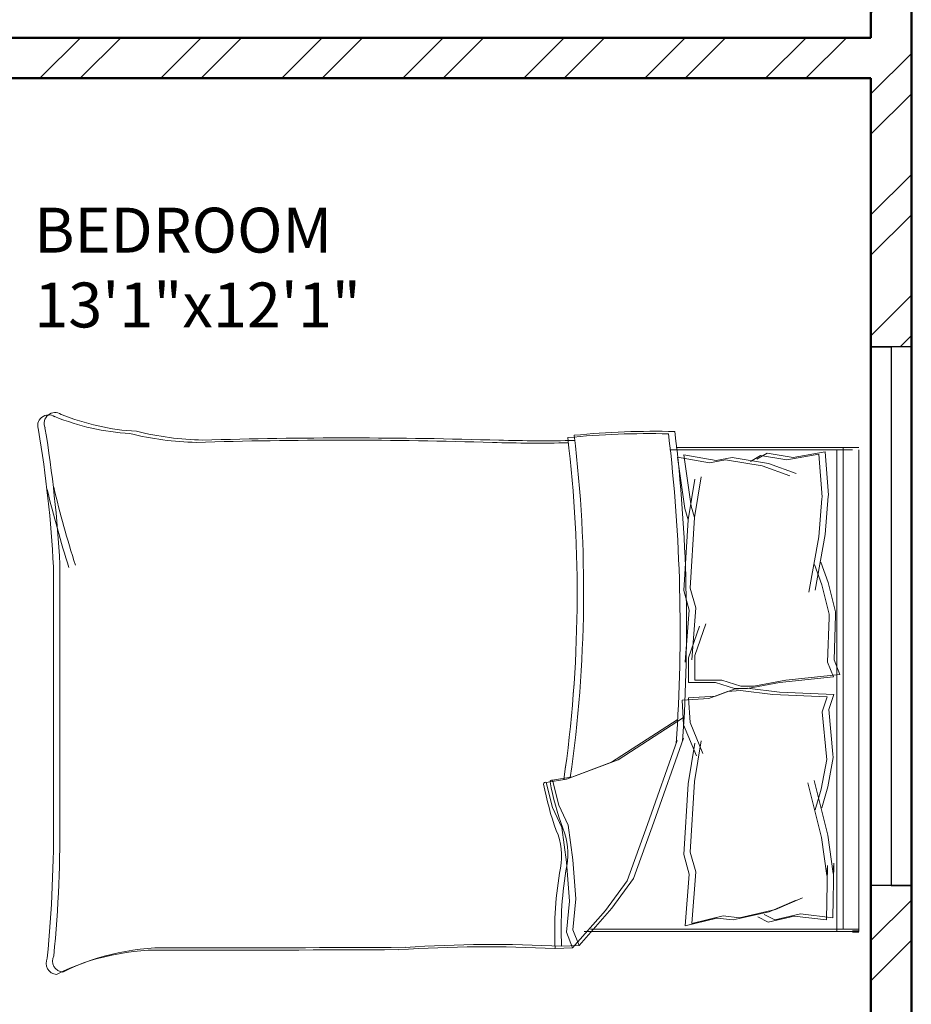
# Model space of a CAD drawing. Units: inches. Extents: x 1901 to 2863, y 888 to 2433.
# Tile 13 of 91: x 2244 to 2343, y 1348 to 1458. Entities that reach past the tile are written whole.
import ezdxf

# ---------------------------------------------------------------- set-up
doc = ezdxf.new("R2010")
doc.units = ezdxf.units.IN
for name, color, linetype, lineweight in [('A-AREA-IDEN', 7, 'Continuous', 18), ('A-FURN', 8, 'Continuous', 18), ('A-GLAZ', 3, 'Continuous', 25), ('A-WALL', 7, 'Continuous', 50), ('A-WALL-PATT', 8, 'Continuous', 13)]:
    doc.layers.add(name, color=color, linetype=linetype, lineweight=lineweight)
doc.styles.get("Standard").update_dxf_attribs({"font": 'arial.ttf'})

# ---------------------------------------------------------------- blocks, each defined once
blk = doc.blocks.new('BED-DOUBLE')
for p, q in [((31.18, 59.32), (27.53, 55.16)), ((31.18, 59.32), (27.53, 55.16)), ((31.9, 59.58), (28.25, 55.42)), ((31.9, 59.58), (28.25, 55.42)), ((33.14, 59.41), (31.18, 59.32, 4.35)), ((33.14, 59.41), (31.18, 59.32, 4.35)), ((31.87, 57.59), (31.18, 59.32)), ((31.87, 57.59), (31.18, 59.32)), ((33.85, 59.67), (31.9, 59.58, 4.35)), ((33.85, 59.67), (31.9, 59.58, 4.35)), ((32.59, 57.85), (31.9, 59.58)), ((32.59, 57.85), (31.9, 59.58)), ((0.03, 57.78), (0.03, 4.12)), ((0.74, 57.78), (30.62, 57.78)), ((0.74, 57.78), (30.62, 57.78)), ((19.35, 57.14), (15.83, 56.27)), ((19.35, 57.14), (15.83, 56.27)), ((18.9, 51.38), (19.35, 57.14)), ((18.9, 51.38), (19.35, 57.14)), ((31.53, 54.12), (31.87, 57.59)), ((31.53, 54.12), (31.87, 57.59)), ((32.24, 54.37), (32.59, 57.85)), ((32.24, 54.37), (32.59, 57.85)), ((2.9, 56.23), (2.79, 50.16)), ((2.9, 56.23), (2.79, 50.16)), ((2.9, 56.23), (6.5, 55.8)), ((2.9, 56.23), (6.5, 55.8)), ((3.61, 56.48), (3.51, 50.42)), ((3.61, 56.48), (3.51, 50.42)), ((3.61, 56.48), (7.22, 56.06)), ((3.61, 56.48), (7.22, 56.06)), ((6.5, 55.8), (9.39, 56.47)), ((6.5, 55.8), (9.39, 56.47)), ((7.22, 56.06), (10.11, 56.73)), ((7.22, 56.06), (10.11, 56.73)), ((13.31, 56.23), (9.3, 55.33)), ((13.31, 56.23), (9.3, 55.33)), ((9.39, 56.47), (10.56, 55.89)), ((9.39, 56.47), (10.56, 55.89)), ((14.02, 56.48), (10.01, 55.58)), ((14.02, 56.48), (10.01, 55.58)), ((10.11, 56.73), (11.28, 56.15)), ((10.11, 56.73), (11.28, 56.15)), ((15.11, 56.01), (13.31, 56.23)), ((15.11, 56.01), (13.31, 56.23)), ((15.83, 56.27), (14.02, 56.48)), ((15.83, 56.27), (14.02, 56.48)), ((18.63, 56.89), (15.11, 56.01)), ((18.63, 56.88), (15.11, 56.01)), ((18.18, 51.12), (18.63, 56.89)), ((18.18, 51.12), (18.63, 56.88)), ((9.3, 55.33), (6.29, 54)), ((9.3, 55.33), (6.29, 54)), ((10.01, 55.58), (7.01, 54.26)), ((10.01, 55.58), (7.01, 54.26)), ((27.53, 55.16), (25.1, 51.86)), ((27.53, 55.16), (25.1, 51.86)), ((28.25, 55.42), (25.81, 52.11)), ((28.25, 55.42), (25.81, 52.11)), ((31.87, 49.77), (31.53, 54.12)), ((31.87, 49.77), (31.53, 54.12)), ((32.59, 50.03), (32.24, 54.37)), ((32.59, 50.03), (32.24, 54.37)), ((25.1, 51.86), (22.84, 45.6)), ((25.1, 51.86), (22.84, 45.6)), ((25.81, 52.11), (23.55, 45.85)), ((25.81, 52.11), (23.55, 45.85)), ((2.79, 50.16), (2.88, 51.29)), ((2.79, 50.16), (2.88, 51.29)), ((2.88, 51.29), (3.47, 47.02)), ((2.88, 51.29), (3.47, 47.02)), ((3.51, 50.42), (3.6, 51.54)), ((3.51, 50.42), (3.6, 51.54)), ((3.6, 51.54), (4.19, 47.28)), ((3.6, 51.54), (4.19, 47.28)), ((18.81, 48.92), (18.18, 51.12)), ((18.81, 48.92), (18.18, 51.12)), ((19.52, 49.18), (18.9, 51.38)), ((19.52, 49.18), (18.9, 51.38)), ((32.39, 45.94), (31.87, 49.77)), ((32.39, 45.94), (31.87, 49.77)), ((33.11, 46.2), (32.59, 50.03)), ((33.11, 46.2), (32.59, 50.03)), ((18.32, 41.05), (18.81, 48.92)), ((18.32, 41.05), (18.81, 48.92)), ((19.04, 41.31), (19.52, 49.18)), ((19.04, 41.31), (19.52, 49.18)), ((4.19, 47.28), (5.71, 41.19)), ((4.19, 47.28), (5.71, 41.19)), ((3.47, 47.02), (4.99, 40.94)), ((3.47, 47.02), (4.99, 40.94)), ((34.15, 43.94), (33.11, 46.2)), ((34.15, 43.94), (33.11, 46.2)), ((22.84, 45.6), (19.54, 36.24)), ((22.84, 45.6), (19.54, 36.24)), ((23.55, 45.85), (20.26, 36.49)), ((23.55, 45.85), (20.26, 36.49)), ((33.44, 43.68), (32.39, 45.94)), ((33.44, 43.68), (32.39, 45.94)), ((4.15, 43.98), (3.48, 41.66)), ((4.15, 43.98), (3.48, 41.66)), ((4.87, 44.23), (4.2, 41.91)), ((4.87, 44.23), (4.2, 41.91)), ((34.85, 41.16), (34.15, 43.94)), ((34.85, 41.16), (34.15, 43.94)), ((89, 16.88), (89, 44.51)), ((89, 16.88), (89, 44.51)), ((89.72, 17.13), (89.72, 44.77)), ((89.72, 17.13), (89.72, 44.77)), ((34.13, 40.9), (33.44, 43.68)), ((34.13, 40.9), (33.44, 43.68)), ((4.2, 41.91), (3.59, 38.62)), ((4.2, 41.91), (3.59, 38.62)), ((3.48, 41.66), (2.87, 38.37)), ((3.48, 41.66), (2.87, 38.37)), ((17.57, 36.53), (18.32, 41.05)), ((17.57, 36.52), (18.32, 41.05)), ((18.29, 36.78), (19.04, 41.31)), ((18.29, 36.78), (19.04, 41.31)), ((27.55, 38.9), (32.59, 40.81)), ((27.55, 38.9), (32.59, 40.81)), ((31.87, 40.55), (34.13, 40.9)), ((31.87, 40.55), (34.13, 40.9)), ((32.59, 40.81), (34.85, 41.16)), ((32.59, 40.81), (34.85, 41.16)), ((26.83, 38.64), (31.87, 40.55)), ((26.83, 38.64), (31.87, 40.55)), ((3.59, 38.62), (3.62, 38.26)), ((3.59, 38.62), (3.62, 38.26)), ((19.54, 33.94), (26.83, 38.64)), ((19.54, 33.94), (26.83, 38.64)), ((20.26, 34.19), (27.55, 38.9)), ((20.26, 34.19), (27.55, 38.9)), ((2.87, 38.37), (2.9, 38.01)), ((2.87, 38.37), (2.9, 38.01)), ((2.9, 38.01), (3.37, 33.03)), ((2.9, 38.01), (3.37, 33.04)), ((3.62, 38.26), (4.09, 33.29)), ((3.62, 38.26), (4.09, 33.29)), ((18.82, 34.49), (17.38, 37.94)), ((18.82, 34.49), (17.38, 37.94)), ((19.54, 34.74), (18.1, 38.19)), ((19.54, 34.74), (18.1, 38.19)), ((18.99, 31.73), (18.82, 34.49)), ((18.99, 31.73), (18.82, 34.49)), ((19.71, 31.99), (19.54, 34.74)), ((19.71, 31.99), (19.54, 34.74)), ((3.37, 33.04), (2.82, 31.37)), ((3.37, 33.03), (2.82, 31.37)), ((4.09, 33.29), (3.54, 31.63)), ((4.09, 33.29), (3.54, 31.63)), ((16.71, 31.8), (19.71, 31.99)), ((16.71, 31.8), (19.71, 31.99)), ((2.82, 31.37), (8.86, 31.1)), ((2.82, 31.37), (8.86, 31.1)), ((3.54, 31.63), (9.58, 31.36)), ((3.54, 31.63), (9.58, 31.36)), ((8.86, 31.1), (12.46, 30.68)), ((8.86, 31.1), (12.46, 30.68)), ((9.58, 31.36), (13.18, 30.93)), ((9.58, 31.36), (13.18, 30.93)), ((12.46, 30.68), (13.92, 30.77)), ((12.46, 30.68), (13.92, 30.77)), ((13.18, 30.93), (14.64, 31.02)), ((13.18, 30.93), (14.64, 31.02)), ((13.92, 30.77), (15.99, 31.55)), ((13.92, 30.77), (15.99, 31.55)), ((14.64, 31.02), (16.71, 31.8)), ((14.64, 31.02), (16.71, 31.8)), ((15.99, 31.55), (18.99, 31.73)), ((15.99, 31.55), (18.99, 31.73)), ((2.13, 29.14), (8.13, 29.78)), ((2.13, 29.14), (8.13, 29.78)), ((2.84, 29.39), (8.85, 30.04)), ((2.84, 29.39), (8.85, 30.04)), ((8.13, 29.78), (11.7, 30.43)), ((8.13, 29.78), (11.7, 30.43)), ((8.85, 30.04), (12.42, 30.69)), ((8.85, 30.04), (12.42, 30.69)), ((11.7, 30.43), (13.16, 30.43)), ((11.7, 30.43), (13.16, 30.43)), ((12.42, 30.69), (13.88, 30.69)), ((12.42, 30.69), (13.88, 30.69)), ((13.16, 30.43), (15.28, 29.78)), ((13.16, 30.43), (15.28, 29.78)), ((13.88, 30.69), (15.99, 30.04)), ((13.88, 30.69), (15.99, 30.04)), ((15.28, 29.78), (18.29, 29.78)), ((15.28, 29.78), (18.29, 29.78)), ((15.99, 30.04), (19, 30.04)), ((15.99, 30.04), (19, 30.04)), ((18.29, 29.78), (18.29, 27.03)), ((18.29, 29.78), (18.29, 27.03)), ((19, 30.04), (19, 27.28)), ((19, 30.04), (19, 27.28)), ((2.78, 27.51), (2.13, 29.14)), ((2.78, 27.51), (2.13, 29.14)), ((3.49, 27.77), (2.84, 29.39)), ((3.49, 27.77), (2.84, 29.39)), ((2.61, 22.52), (2.78, 27.51)), ((2.61, 22.52), (2.78, 27.51)), ((3.33, 22.78), (3.49, 27.77)), ((3.33, 22.78), (3.49, 27.77)), ((18.18, 21.73), (18.63, 27.49)), ((18.18, 21.73), (18.63, 27.49)), ((18.9, 21.98), (19.35, 27.75)), ((18.9, 21.98), (19.35, 27.74)), ((18.29, 27.03), (17.06, 23.49)), ((18.29, 27.03), (17.06, 23.5)), ((19, 27.28), (17.78, 23.75)), ((19, 27.28), (17.78, 23.75)), ((2.61, 22.16), (2.61, 22.52)), ((2.61, 22.16), (2.61, 22.52)), ((3.42, 18.91), (2.61, 22.16)), ((3.42, 18.91), (2.61, 22.16)), ((3.33, 22.42), (3.33, 22.78)), ((3.33, 22.42), (3.33, 22.78)), ((4.14, 19.17), (3.33, 22.42)), ((4.14, 19.17), (3.33, 22.42)), ((19.52, 19.78), (18.9, 21.98)), ((19.52, 19.78), (18.9, 21.98)), ((18.81, 19.53), (18.18, 21.73)), ((18.81, 19.53), (18.18, 21.73)), ((4.47, 13.81), (5.6, 19.98)), ((4.47, 13.81), (5.6, 19.98)), ((19.04, 11.91), (19.52, 19.78)), ((19.04, 11.91), (19.52, 19.78)), ((4.24, 16.64), (3.42, 18.91)), ((4.24, 16.64), (3.42, 18.91)), ((3.75, 13.56), (4.89, 19.73)), ((3.75, 13.56), (4.89, 19.73)), ((4.95, 16.9), (4.14, 19.17)), ((4.95, 16.9), (4.14, 19.17)), ((18.32, 11.66), (18.81, 19.53)), ((18.32, 11.66), (18.81, 19.53)), ((3.42, 9.27), (3.75, 13.56)), ((3.42, 9.27), (3.75, 13.56)), ((4.14, 9.52), (4.47, 13.81)), ((4.14, 9.52), (4.47, 13.81)), ((17.57, 7.13), (18.32, 11.66)), ((17.57, 7.13), (18.32, 11.66)), ((18.29, 7.38), (19.04, 11.91)), ((18.29, 7.39), (19.04, 11.91)), ((18.32, 11.66), (18.68, 10.38)), ((18.32, 11.66), (18.68, 10.38)), ((19.04, 11.91), (19.4, 10.64)), ((19.04, 11.91), (19.4, 10.64)), ((18.68, 10.38), (19.5, 4.66)), ((18.68, 10.38), (19.5, 4.66)), ((19.4, 10.64), (20.21, 4.92)), ((19.4, 10.64), (20.21, 4.92)), ((3.4, 9.15), (3.42, 9.27)), ((3.4, 9.15), (3.42, 9.27)), ((3.77, 4.34), (3.4, 9.15)), ((3.77, 4.34), (3.4, 9.15)), ((4.12, 9.4), (4.14, 9.52)), ((4.12, 9.4), (4.14, 9.52)), ((4.49, 4.6), (4.12, 9.4)), ((4.49, 4.6), (4.12, 9.4)), ((10.08, 5.63), (7, 6.77)), ((10.08, 5.63), (7, 6.77)), ((10.8, 5.89), (7.71, 7.03)), ((10.8, 5.89), (7.71, 7.03)), ((14.14, 4.99), (10.08, 5.63)), ((14.14, 4.99), (10.08, 5.63)), ((14.86, 5.24), (10.8, 5.89)), ((14.86, 5.24), (10.8, 5.89)), ((16.64, 5.57), (14.86, 5.24)), ((16.64, 5.57), (14.86, 5.24)), ((20.21, 4.92), (16.64, 5.57)), ((20.21, 4.92), (16.64, 5.57)), ((3.75, 4.34), (7.32, 4.99)), ((3.75, 4.34), (7.32, 4.99)), ((4.47, 4.59), (8.04, 5.24)), ((4.47, 4.59), (8.04, 5.24)), ((7.32, 4.99), (10.24, 4.5)), ((7.32, 4.99), (10.24, 4.5)), ((8.04, 5.24), (10.96, 4.75)), ((8.04, 5.24), (10.96, 4.76)), ((10.24, 4.5), (11.38, 5.15)), ((10.24, 4.5), (11.38, 5.15)), ((10.96, 4.76), (12.1, 5.4)), ((10.96, 4.75), (12.1, 5.4)), ((15.92, 5.31), (14.14, 4.99)), ((15.92, 5.31), (14.14, 4.99)), ((19.5, 4.66), (15.92, 5.31)), ((19.5, 4.66), (15.92, 5.31))]:
    blk.add_line(p, q)
for centre, radius, start, end in [((77.84, 85.73), 25.9, 267.4714, 296.4681), ((77.84, 85.73), 25.9, 267.4714, 296.4681), ((89.3, 61.31), 1.24, 332.6588, 86.02), ((89.3, 61.31), 1.24, 332.6588, 86.02), ((77.12, 85.47), 25.9, 267.4714, 296.4681), ((77.12, 85.47), 25.9, 267.4714, 296.4681), ((88.58, 61.05), 1.24, 332.6588, 86.02), ((88.58, 61.05), 1.24, 332.6588, 86.02), ((238.36, 46.17), 149.37, 174.4998, 180.6351), ((238.36, 46.17), 149.37, 174.4998, 180.6351), ((239.08, 46.42), 149.37, 174.4998, 180.6351), ((239.08, 46.42), 149.37, 174.4998, 180.6351), ((-7.45, 57.59), 40.62, 349.8763, 2.5657), ((-7.45, 57.59), 40.62, 349.8763, 2.5657), ((40.8, 204.6), 145.39, 266.9791, 273.8365), ((40.8, 204.6), 145.39, 266.9791, 273.8365), ((-6.73, 57.85), 40.62, 349.8763, 2.5657), ((-6.73, 57.85), 40.62, 349.8763, 2.5657), ((41.52, 204.86), 145.39, 266.9791, 273.8365), ((41.52, 204.86), 145.39, 266.9791, 273.8365), ((76.17, -5062.23), 5121.82, 90.00217, 90.28689), ((76.17, -5062.23), 5121.82, 90.00217, 90.28689), ((76.89, -5061.97), 5121.82, 90.00217, 90.28689), ((76.89, -5061.97), 5121.82, 90.00217, 90.28689), ((39.4, 49.08), 6.99, 168.6608, 203.7384), ((39.4, 49.08), 6.99, 168.6608, 203.7384), ((40.11, 49.33), 6.99, 168.6608, 203.7384), ((40.11, 49.33), 6.99, 168.6608, 203.7384), ((1.69, 34.94), 33.29, 10.6617, 19.8806), ((1.69, 34.94), 33.29, 10.6617, 19.8806), ((2.41, 35.2), 33.29, 10.6617, 19.8806), ((2.41, 35.2), 33.29, 10.6617, 19.8806), ((175.53, 19.9), 144.86, 171.7845, 186.9006), ((175.53, 19.9), 144.86, 171.7845, 186.9006), ((176.25, 20.16), 144.86, 171.7845, 186.9006), ((176.25, 20.15), 144.86, 171.7845, 186.9006), ((34.2, 41.1), 0.207, 250.2464, 1.1377), ((34.2, 41.1), 0.207, 250.2464, 1.1377), ((34.92, 41.35), 0.207, 250.2464, 1.1377), ((34.92, 41.35), 0.207, 250.2464, 1.1377), ((204.43, 23.94), 185.22, 176.0865, 186.7821), ((204.43, 23.94), 185.22, 176.0865, 186.7821), ((205.14, 24.2), 185.22, 176.0865, 186.7821), ((205.14, 24.2), 185.22, 176.0865, 186.7821), ((225.52, 24.02), 136.7, 182.9958, 189.4091), ((225.52, 24.02), 136.7, 182.9958, 189.4091), ((226.23, 24.28), 136.7, 182.9958, 189.4091), ((226.23, 24.28), 136.7, 182.9958, 189.4091), ((35.74, -187.62), 190.99, 88.4762, 91.0082), ((35.74, -187.62), 190.99, 88.4762, 91.0082), ((57.57, 544.55), 541.51, 268.2277, 271.7185), ((57.57, 544.55), 541.51, 268.2277, 271.7185), ((22.59, 95.58), 93.53, 268.7218, 275.604), ((22.59, 95.58), 93.53, 268.7218, 275.604), ((23.31, 95.84), 93.53, 268.7218, 275.604), ((23.31, 95.84), 93.53, 268.7218, 275.604), ((35.03, -187.88), 190.99, 88.4762, 91.0082), ((35.03, -187.88), 190.99, 88.4762, 91.0082), ((56.85, 544.3), 541.51, 268.2277, 271.7185), ((56.85, 544.3), 541.51, 268.2277, 271.7185), ((72.46, -30.24), 33.27, 76.0648, 88.9113), ((72.46, -30.24), 33.27, 76.0648, 88.9113), ((73.18, -29.98), 33.27, 76.0648, 88.9113), ((73.18, -29.98), 33.27, 76.0648, 88.9113), ((79.65, -24.1), 26.45, 67.9751, 86.652), ((79.65, -24.1), 26.45, 67.9751, 86.652), ((78.93, -24.35), 26.45, 67.9751, 86.652), ((78.93, -24.35), 26.45, 67.9751, 86.652), ((89.53, 1.18), 1.22, 236.1736, 23.4781), ((89.53, 1.18), 1.22, 236.1736, 23.4781), ((90.25, 1.44), 1.22, 236.1736, 23.4781), ((90.25, 1.44), 1.22, 236.1736, 23.4781)]:
    blk.add_arc(centre, radius, start, end)
blk = doc.blocks.new('WIN-60')
for p, q in [((0, 4.5), (0, 0)), ((60, 2.25), (60, 4.5)), ((60, 4.5), (60, 0)), ((0, 0), (0, 2.25)), ((0, 2.25), (60, 2.25))]:
    blk.add_line(p, q)

msp = doc.modelspace()

# ---------------------------------------------------------------- hatches: boundary and pattern name
at = {"layer": 'A-WALL-PATT'}
h = msp.add_hatch(dxfattribs=at)
h.set_pattern_fill('ANSI32', color=256)
h.paths.add_polyline_path([(2192.5, 2274.13), (2141.26, 2274.13), (2141.26, 2269.63), (2192.5, 2269.63)])
h.paths.add_polyline_path([(2259.93, 2274.13), (2216.5, 2274.13), (2216.5, 2269.63), (2255.43, 2269.63), (2255.43, 2214.63), (2250.81, 2214.63), (2250.81, 2210.13), (2259.93, 2210.13), (2259.93, 2215.13), (2271.76, 2215.13), (2271.76, 2217.38), (2271.76, 2219.63), (2259.93, 2219.63)])
h.paths.add_polyline_path([(2171.43, 2269.63), (2166.93, 2269.63), (2166.93, 2219.63), (2121.24, 2219.63), (2121.24, 2215.13), (2166.93, 2215.13), (2166.93, 2083.13), (2161.81, 2083.13), (2161.81, 2078.63), (2171.43, 2078.63), (2177, 2078.63), (2177, 2080.88), (2177, 2083.13), (2171.43, 2083.13), (2171.43, 2210.13), (2230.91, 2210.13), (2230.91, 2212.38), (2230.91, 2214.63), (2171.43, 2214.63)])
h.paths.add_polyline_path([(2117.26, 2274.13), (2089.43, 2274.13), (2089.43, 2219.63), (2081.14, 2219.63), (2081.14, 2215.13), (2089.43, 2215.13), (2098, 2215.13), (2098, 2217.38), (2098, 2219.63), (2093.93, 2219.63), (2093.93, 2269.63), (2117.26, 2269.63), (2117.26, 2271.88)])
h.paths.add_polyline_path([(2343.43, 2219.63), (2329.29, 2219.63), (2329.29, 2215.13), (2338.93, 2215.13), (2338.93, 2184.74), (2343.43, 2184.74)])
h.paths.add_polyline_path([(2338.93, 2083.13), (2329.29, 2083.13), (2208.97, 2083.13), (2208.97, 2078.63), (2338.93, 2078.63)])
h.paths.add_polyline_path([(2343.43, 2136.74), (2338.93, 2136.74), (2338.93, 1872.63), (2343.43, 1872.63)])
h.paths.add_polyline_path([(2343.43, 1863.63), (2397.68, 1863.63), (2397.68, 1821.63), (2384.14, 1821.63), (2384.14, 1812.63), (2418.33, 1812.63), (2418.33, 1817.13), (2418.33, 1821.63), (2406.68, 1821.63), (2406.68, 1863.63), (2459.5, 1863.63), (2459.5, 1821.63), (2447.14, 1821.63), (2447.14, 1812.63), (2459.5, 1812.63), (2468.5, 1812.63), (2468.5, 1872.63), (2394.43, 1872.63), (2334.43, 1872.63), (2334.43, 1812.63), (2343.43, 1812.63), (2353.25, 1812.63), (2353.25, 1821.63), (2343.43, 1821.63)])
h.paths.add_polyline_path([(2510.01, 1872.63), (2468.5, 1872.63), (2468.5, 1868.13), (2510.01, 1868.13)])
h.paths.add_polyline_path([(2514.01, 1817.13), (2468.5, 1817.13), (2468.5, 1812.63), (2482.11, 1812.63), (2482.11, 1800.61), (2486.61, 1800.61), (2486.61, 1812.63), (2514.01, 1812.63)])
h.paths.add_polyline_path([(2299.25, 1814.88), (2299.25, 1817.13), (2295.93, 1817.13), (2295.93, 1854.17), (2293.68, 1854.17), (2291.43, 1854.17), (2291.43, 1817.13), (2266.11, 1817.13), (2266.11, 1812.63), (2299.25, 1812.63)])
h.paths.add_polyline_path([(2218.11, 1817.13), (2206.46, 1817.13), (2171.43, 1817.13), (2171.43, 1949.13), (2190.1, 1949.13), (2190.1, 1953.63), (2163.47, 1953.63), (2163.47, 1949.13), (2166.93, 1949.13), (2166.93, 1817.13), (2114.3, 1817.13), (2114.3, 1812.63), (2218.11, 1812.63)])
h.paths.add_polyline_path([(2029.43, 1970.92), (2024.93, 1970.92), (2024.93, 1912.72), (2029.43, 1912.72)])
h.paths.add_polyline_path([(2132.3, 1953.63), (2113.93, 1953.63), (2113.93, 1975.89), (2111.68, 1975.89), (2109.43, 1975.89), (2109.43, 1953.63), (2029.43, 1953.63), (2029.43, 1949.13), (2132.3, 1949.13)])
h.paths.add_polyline_path([(2029.43, 1853.61), (2029.31, 1853.61), (2029.31, 1853.61), (2029.43, 1853.61), (2029.43, 1864.72), (2024.93, 1864.72), (2024.93, 1812.63), (2066.3, 1812.63), (2066.3, 1814.88), (2066.3, 1817.13), (2029.43, 1817.13)])
h.paths.add_polyline_path([(2122.93, 2010.09), (2120.68, 2010.09), (2118.43, 2010.09), (2118.43, 2006.13), (2029.43, 2006.13), (2029.43, 2001.63), (2109.43, 2001.63), (2109.43, 1998.04), (2113.93, 1998.04), (2113.93, 2001.63), (2122.93, 2001.63)])
h.paths.add_polyline_path([(2029.43, 2031.38), (2024.93, 2031.38), (2024.93, 1994.92), (2027.18, 1994.92), (2029.43, 1994.92)])
h.paths.add_polyline_path([(2029.43, 2136.74), (2024.93, 2136.74), (2024.93, 2067.38), (2027.18, 2067.38), (2029.43, 2067.38)])
h.paths.add_polyline_path([(2125.62, 2083.13), (2029.43, 2083.13), (2029.43, 2078.63), (2118.43, 2078.63), (2118.43, 2030.71), (2122.93, 2030.71), (2122.93, 2078.63), (2125.62, 2078.63)])
h.paths.add_polyline_path([(2029.43, 2215.13), (2040.47, 2215.13), (2040.47, 2217.38), (2040.47, 2219.63), (2024.93, 2219.63), (2024.93, 2184.74), (2029.43, 2184.74), (2029.43, 2187.78)])
h.paths.add_polyline_path([(2686.43, 2274.13), (2659.28, 2274.13), (2659.28, 2269.63), (2681.93, 2269.63), (2681.93, 2219.63), (2676.82, 2219.63), (2676.82, 2215.13), (2681.93, 2215.13), (2697.01, 2215.13), (2697.01, 2217.38), (2697.01, 2219.63), (2686.43, 2219.63)])
h.paths.add_polyline_path([(2609.93, 2269.63), (2635.28, 2269.63), (2635.28, 2274.13), (2571.43, 2274.13), (2571.43, 2269.63), (2605.43, 2269.63), (2605.43, 2214.63), (2549.1, 2214.63), (2549.1, 2210.13), (2605.43, 2210.13), (2605.43, 2083.13), (2601.01, 2083.13), (2601.01, 2080.88), (2601.01, 2078.63), (2609.93, 2078.63), (2616.16, 2078.63), (2616.16, 2080.88), (2616.16, 2083.13), (2609.93, 2083.13), (2609.93, 2215.13), (2651.46, 2215.13), (2651.46, 2217.38), (2651.46, 2219.63), (2609.93, 2219.63)])
h.paths.add_polyline_path([(2521.43, 2269.63), (2547.43, 2269.63), (2547.43, 2271.88), (2547.43, 2274.13), (2516.93, 2274.13), (2516.93, 2219.63), (2506.41, 2219.63), (2506.41, 2215.13), (2516.93, 2215.13), (2516.93, 2210.13), (2525.4, 2210.13), (2525.4, 2212.38), (2525.4, 2214.63), (2521.43, 2214.63)])
h.paths.add_polyline_path([(2456.01, 2219.63), (2439.43, 2219.63), (2439.43, 2187.89), (2443.93, 2187.89), (2443.93, 2215.13), (2456.01, 2215.13)])
h.paths.add_polyline_path([(2752.93, 2219.63), (2739.48, 2219.63), (2739.48, 2215.13), (2748.43, 2215.13), (2748.43, 2187.89), (2752.93, 2187.89)])
h.paths.add_polyline_path([(2752.93, 2139.89), (2748.43, 2139.89), (2748.43, 2083.13), (2648.42, 2083.13), (2648.42, 2078.63), (2654.93, 2078.63), (2654.93, 2039.44), (2659.43, 2039.44), (2659.43, 2078.63), (2748.43, 2078.63), (2748.43, 2063.43), (2752.93, 2063.43)])
h.paths.add_polyline_path([(2752.93, 2010.63), (2659.43, 2010.63), (2659.43, 2015.65), (2654.93, 2015.65), (2654.93, 2010.63), (2605.43, 2010.63), (2605.43, 1920.97), (2609.93, 1920.97), (2609.93, 2006.13), (2748.43, 2006.13), (2748.43, 1982.47), (2752.93, 1982.47)])
h.paths.add_polyline_path([(2752.93, 2027.43), (2748.43, 2027.43), (2748.43, 2010.63), (2752.93, 2010.63)])
h.paths.add_polyline_path([(2748.43, 1886.13), (2609.93, 1886.13), (2609.93, 1889.72), (2605.43, 1889.72), (2605.43, 1861.26), (2609.93, 1861.26), (2609.93, 1881.63), (2748.43, 1881.63)])
h.paths.add_polyline_path([(2456.86, 2228.83), (2498.4, 2228.83), (2498.4, 2247.49), (2456.86, 2247.49)], flags=9)
h.paths.add_polyline_path([(2038.6, 2237.42), (2080.17, 2237.42), (2080.17, 2256.08), (2038.6, 2256.08)], flags=9)
h.paths.add_polyline_path([(2292.01, 1062.39), (2539.93, 1062.39), (2539.93, 1099.49), (2292.01, 1099.49)], flags=9)
h.paths.add_polyline_path([(2424.91, 1832.25), (2448.51, 1832.25), (2448.51, 1846.68), (2424.91, 1846.68)], flags=25)
h.paths.add_polyline_path([(2359.08, 1832.25), (2382.68, 1832.25), (2382.68, 1846.68), (2359.08, 1846.68)], flags=25)
h.paths.add_polyline_path([(2352.9, 1684.8), (2367.54, 1684.8), (2367.54, 1697.17), (2352.9, 1697.17)], flags=9)
h.paths.add_polyline_path([(2079.29, 1755.83), (2169.02, 1755.83), (2169.02, 1774.37), (2079.29, 1774.37)], flags=9)
h.paths.add_polyline_path([(2404.09, 1373.86), (2404.09, 1463.59), (2385.54, 1463.59), (2385.54, 1373.86)], flags=9)
h.paths.add_polyline_path([(2268.09, 2236.37), (2309.64, 2236.37), (2309.64, 2255.03), (2268.09, 2255.03)], flags=9)
h.paths.add_polyline_path([(2575.96, 1700.95), (2665.7, 1700.95), (2665.7, 1719.5), (2575.96, 1719.5)], flags=9)
h.paths.add_polyline_path([(2302.96, 1878.47), (2329.52, 1878.47), (2329.52, 1888.78), (2302.96, 1888.78)], flags=9)
h.paths.add_polyline_path([(2097.42, 2240.58), (2126.57, 2240.58), (2126.57, 2259.23), (2097.42, 2259.23)], flags=9)
h.paths.add_polyline_path([(2208.72, 2246.12), (2237.88, 2246.12), (2237.88, 2264.78), (2208.72, 2264.78)], flags=9)
h.paths.add_polyline_path([(2038.15, 1925.96), (2076.99, 1925.96), (2076.99, 1944.62), (2038.15, 1944.62)], flags=9)
h.paths.add_polyline_path([(2239.14, 1926.67), (2288.46, 1926.67), (2288.46, 1945.33), (2239.14, 1945.33)], flags=9)
h.paths.add_polyline_path([(2175.43, 2007.33), (2212.36, 2007.33), (2212.36, 2025.99), (2175.43, 2025.99)], flags=9)
h.paths.add_polyline_path([(2225.03, 2091.79), (2263.87, 2091.79), (2263.87, 2110.45), (2225.03, 2110.45)], flags=9)
h.paths.add_polyline_path([(2035.4, 2098.48), (2074.24, 2098.48), (2074.24, 2117.14), (2035.4, 2117.14)], flags=9)
h.paths.add_polyline_path([(2050.1, 2029.21), (2083.26, 2029.21), (2083.26, 2047.87), (2050.1, 2047.87)], flags=9)
h.paths.add_polyline_path([(2069.68, 1956.72), (2098.83, 1956.72), (2098.83, 1975.38), (2069.68, 1975.38)], flags=25)
h.paths.add_polyline_path([(2328.62, 1753.34), (2361.66, 1753.34), (2361.66, 1771.99), (2328.62, 1771.99)], flags=9)
h.paths.add_polyline_path([(2395.16, 2060.89), (2395.16, 2140.65), (2378.68, 2140.65), (2378.68, 2060.89)], flags=9)
h.paths.add_polyline_path([(2463.73, 2059.02), (2492.89, 2059.02), (2492.89, 2077.68), (2463.73, 2077.68)], flags=9)
h.paths.add_polyline_path([(2458.03, 2181.54), (2496.87, 2181.54), (2496.87, 2200.19), (2458.03, 2200.19)], flags=9)
h.paths.add_polyline_path([(2527.58, 2243.07), (2556.73, 2243.07), (2556.73, 2261.73), (2527.58, 2261.73)], flags=9)
h.paths.add_polyline_path([(2694.46, 2232.77), (2736.03, 2232.77), (2736.03, 2251.42), (2694.46, 2251.42)], flags=9)
h.paths.add_polyline_path([(2637.82, 2249.22), (2666.98, 2249.22), (2666.98, 2267.88), (2637.82, 2267.88)], flags=9)
h.paths.add_polyline_path([(2623.69, 2183.54), (2662.53, 2183.54), (2662.53, 2202.2), (2623.69, 2202.2)], flags=9)
h.paths.add_polyline_path([(2691.97, 2021.5), (2725.12, 2021.5), (2725.12, 2040.16), (2691.97, 2040.16)], flags=9)
h.paths.add_polyline_path([(2621.04, 1975.91), (2662.34, 1975.91), (2662.34, 1994.57), (2621.04, 1994.57)], flags=25)
h.paths.add_polyline_path([(2479.03, 1927.62), (2519.84, 1927.62), (2519.84, 1946.28), (2479.03, 1946.28)], flags=9)
h.paths.add_polyline_path([(2670.94, 1849.08), (2716.01, 1849.08), (2716.01, 1867.73), (2670.94, 1867.73)], flags=9)
h.paths.add_polyline_path([(2523.61, 1782.96), (2550.17, 1782.96), (2550.17, 1793.26), (2523.61, 1793.26)], flags=9)
h.paths.add_polyline_path([(2450.84, 1207.33), (2492.39, 1207.33), (2492.39, 1225.99), (2450.84, 1225.99)], flags=9)
h.paths.add_polyline_path([(2527.75, 1203.84), (2556.91, 1203.84), (2556.91, 1222.5), (2527.75, 1222.5)], flags=9)
h.paths.add_polyline_path([(2639.11, 1207.2), (2668.27, 1207.2), (2668.27, 1225.86), (2639.11, 1225.86)], flags=9)
h.paths.add_polyline_path([(2692.59, 1218.97), (2734.17, 1218.97), (2734.17, 1237.62), (2692.59, 1237.62)], flags=9)
h.paths.add_polyline_path([(2669.27, 1366.33), (2708.11, 1366.33), (2708.11, 1384.99), (2669.27, 1384.99)], flags=9)
h.paths.add_polyline_path([(2463.31, 1358.03), (2502.15, 1358.03), (2502.15, 1376.69), (2463.31, 1376.69)], flags=9)
h.paths.add_polyline_path([(2494.72, 1449.96), (2531.65, 1449.96), (2531.65, 1468.62), (2494.72, 1468.62)], flags=9)
h.paths.add_polyline_path([(2675.57, 1422.16), (2708.72, 1422.16), (2708.72, 1440.81), (2675.57, 1440.81)], flags=9)
h.paths.add_polyline_path([(2685.63, 1493.89), (2714.79, 1493.89), (2714.79, 1512.55), (2685.63, 1512.55)], flags=9)
h.paths.add_polyline_path([(2686.8, 1529.91), (2725.65, 1529.91), (2725.65, 1548.57), (2686.8, 1548.57)], flags=9)
h.paths.add_polyline_path([(2503.65, 1537.99), (2552.97, 1537.99), (2552.97, 1556.65), (2503.65, 1556.65)], flags=9)
h.paths.add_polyline_path([(2291.71, 1643.5), (2318.28, 1643.5), (2318.28, 1653.81), (2291.71, 1653.81)], flags=9)
h.paths.add_polyline_path([(2450.63, 1610.52), (2477.19, 1610.52), (2477.19, 1620.82), (2450.63, 1620.82)], flags=9)
h.paths.add_polyline_path([(2359.99, 1551.81), (2422.25, 1551.81), (2422.25, 1562.12), (2359.99, 1562.12)], flags=9)
h.paths.add_polyline_path([(2280.11, 1249.01), (2321.65, 1249.01), (2321.65, 1267.66), (2280.11, 1267.66)], flags=9)
h.paths.add_polyline_path([(2164.06, 1274.23), (2193.22, 1274.23), (2193.22, 1292.89), (2164.06, 1292.89)], flags=9)
h.paths.add_polyline_path([(2118.21, 1277.69), (2151.25, 1277.69), (2151.25, 1296.35), (2118.21, 1296.35)], flags=9)
h.paths.add_polyline_path([(2031.95, 1268.53), (2073.52, 1268.53), (2073.52, 1287.19), (2031.95, 1287.19)], flags=9)
h.paths.add_polyline_path([(2050.2, 1409.08), (2089.04, 1409.08), (2089.04, 1427.74), (2050.2, 1427.74)], flags=9)
h.paths.add_polyline_path([(2243.74, 1421.03), (2282.58, 1421.03), (2282.58, 1439.69), (2243.74, 1439.69)], flags=9)
h.paths.add_polyline_path([(2190.75, 1509.77), (2231.56, 1509.77), (2231.56, 1528.43), (2190.75, 1528.43)], flags=9)
h.paths.add_polyline_path([(2058.39, 1475.42), (2091.55, 1475.42), (2091.55, 1494.07), (2058.39, 1494.07)], flags=9)
h.paths.add_polyline_path([(2062.45, 1553.09), (2091.6, 1553.09), (2091.6, 1571.75), (2062.45, 1571.75)], flags=9)
h.paths.add_polyline_path([(2219.52, 1590.37), (2266.15, 1590.37), (2266.15, 1609.02), (2219.52, 1609.02)], flags=9)
h.paths.add_polyline_path([(2041.07, 1584.19), (2079.91, 1584.19), (2079.91, 1602.85), (2041.07, 1602.85)], flags=9)
h = msp.add_hatch(dxfattribs=at)
h.set_pattern_fill('ANSI32', color=256)
h.paths.add_polyline_path([(2443.93, 2139.89), (2439.43, 2139.89), (2439.43, 2069.35), (2441.68, 2069.35), (2443.93, 2069.35), (2443.93, 2078.63), (2521.93, 2078.63), (2521.93, 2075.07), (2524.18, 2075.07), (2526.43, 2075.07), (2526.43, 2078.63), (2571.75, 2078.63), (2571.75, 2080.88), (2571.75, 2083.13), (2443.93, 2083.13)])
h.paths.add_polyline_path([(2526.43, 2054.63), (2524.18, 2054.63), (2521.93, 2054.63), (2521.93, 2030.63), (2443.93, 2030.63), (2443.93, 2045.35), (2439.43, 2045.35), (2439.43, 1983.87), (2443.93, 1983.87), (2443.93, 2026.13), (2521.93, 2026.13), (2526.43, 2026.13)])
h.paths.add_polyline_path([(2443.93, 1923.87), (2439.43, 1923.87), (2439.43, 1872.63), (2443.93, 1872.63)])
h.paths.add_polyline_path([(2636.23, 1766.13), (2609.93, 1766.13), (2609.93, 1779.79), (2605.43, 1779.79), (2605.43, 1766.13), (2486.61, 1766.13), (2486.61, 1770.67), (2482.11, 1770.67), (2482.11, 1766.13), (2482.11, 1761.63), (2636.23, 1761.63), (2636.23, 1763.88)])
h.paths.add_polyline_path([(2519.54, 1663.38), (2519.54, 1665.63), (2494.93, 1665.63), (2481.83, 1665.63), (2481.83, 1663.38), (2481.83, 1661.13), (2490.43, 1661.13), (2490.43, 1640.16), (2494.93, 1640.16), (2494.93, 1661.13), (2519.54, 1661.13)])
h.paths.add_polyline_path([(2443.93, 1712.13), (2443.93, 1716.63), (2414.46, 1716.63), (2414.46, 1712.13), (2439.43, 1712.13), (2439.43, 1545.51), (2443.93, 1545.51), (2443.93, 1661.13), (2448.47, 1661.13), (2448.47, 1665.63), (2443.93, 1665.63)])
h.paths.add_polyline_path([(2343.43, 1712.13), (2365.52, 1712.13), (2365.52, 1714.38), (2365.52, 1716.63), (2333.87, 1716.63), (2333.87, 1714.38), (2333.87, 1712.13), (2338.93, 1712.13), (2338.93, 1575.63), (2338.93, 1545.51), (2343.43, 1545.51), (2343.43, 1547.51), (2343.43, 1580.13)])
h.paths.add_polyline_path([(2752.93, 1665.63), (2579.54, 1665.63), (2579.54, 1661.13), (2615.93, 1661.13), (2615.93, 1529.13), (2598.93, 1529.13), (2598.93, 1524.63), (2623.13, 1524.63), (2623.13, 1526.88), (2623.13, 1529.13), (2620.43, 1529.13), (2620.43, 1661.13), (2748.43, 1661.13), (2748.43, 1633.5), (2752.93, 1633.5)])
h.paths.add_polyline_path([(2752.93, 1419.93), (2748.43, 1419.93), (2748.43, 1400.13), (2659.43, 1400.13), (2659.43, 1444.33), (2657.18, 1444.33), (2654.93, 1444.33), (2654.93, 1400.13), (2643.65, 1400.13), (2643.65, 1395.63), (2748.43, 1395.63), (2748.43, 1364.04), (2752.93, 1364.04)])
h.paths.add_polyline_path([(2752.93, 1492.88), (2748.43, 1492.88), (2748.43, 1476.63), (2667.43, 1476.63), (2667.43, 1479.71), (2665.18, 1479.71), (2662.93, 1479.71), (2662.93, 1476.63), (2654.93, 1476.63), (2654.93, 1469.54), (2659.43, 1469.54), (2659.43, 1472.13), (2748.43, 1472.13), (2748.43, 1455.93), (2752.93, 1455.93)])
h.paths.add_polyline_path([(2752.93, 1304.04), (2748.43, 1304.04), (2748.43, 1263.63), (2738.66, 1263.63), (2738.66, 1259.13), (2752.93, 1259.13)])
h.paths.add_polyline_path([(2685.93, 1259.13), (2695.49, 1259.13), (2695.49, 1261.38), (2695.49, 1263.63), (2677.84, 1263.63), (2677.84, 1261.38), (2677.84, 1259.13), (2681.43, 1259.13), (2681.43, 1203.63), (2653.28, 1203.63), (2653.28, 1199.13), (2685.93, 1199.13), (2685.93, 1203.63)])
h.paths.add_polyline_path([(2609.43, 1395.63), (2611.85, 1395.63), (2611.85, 1400.13), (2598.89, 1400.13), (2598.89, 1397.88), (2598.89, 1395.63), (2604.93, 1395.63), (2604.93, 1268.13), (2554.73, 1268.13), (2554.73, 1265.88), (2554.73, 1263.63), (2604.93, 1263.63), (2604.93, 1203.63), (2571.31, 1203.63), (2571.31, 1199.13), (2604.93, 1199.13), (2629.28, 1199.13), (2629.28, 1201.38), (2629.28, 1203.63), (2609.43, 1203.63), (2609.43, 1258.63), (2609.43, 1259.13), (2654.8, 1259.13), (2654.8, 1263.63), (2609.43, 1263.63)])
h.paths.add_polyline_path([(2443.93, 1304.04), (2439.43, 1304.04), (2439.43, 1259.13), (2443.93, 1259.13), (2456.16, 1259.13), (2456.16, 1261.38), (2456.16, 1263.63), (2443.93, 1263.63)])
h.paths.add_polyline_path([(2525.43, 1263.63), (2531.78, 1263.63), (2531.78, 1268.13), (2520.93, 1268.13), (2520.93, 1263.63), (2511.41, 1263.63), (2511.41, 1259.13), (2520.93, 1259.13), (2520.93, 1199.13), (2547.31, 1199.13), (2547.31, 1201.38), (2547.31, 1203.63), (2525.43, 1203.63)])
h.paths.add_polyline_path([(2443.93, 1434.84), (2439.43, 1434.84), (2439.43, 1364.04), (2441.68, 1364.04), (2443.93, 1364.04)])
h.paths.add_polyline_path([(2567.13, 1400.13), (2443.93, 1400.13), (2443.93, 1395.63), (2567.13, 1395.63)])
h.paths.add_polyline_path([(2443.93, 1545.51), (2439.43, 1545.51), (2439.43, 1494.84), (2443.93, 1494.84)])
h.paths.add_polyline_path([(2494.93, 1553.35), (2492.68, 1553.35), (2490.43, 1553.35), (2490.43, 1524.63), (2494.93, 1524.63), (2525.94, 1524.63), (2525.94, 1526.88), (2525.94, 1529.13), (2494.93, 1529.13)])
h.paths.add_polyline_path([(2752.93, 1573.5), (2748.43, 1573.5), (2748.43, 1529.13), (2657.76, 1529.13), (2657.76, 1524.63), (2662.93, 1524.63), (2662.93, 1498.63), (2667.43, 1498.63), (2667.43, 1524.63), (2748.43, 1524.63), (2748.43, 1516.88), (2752.93, 1516.88)])
h.paths.add_polyline_path([(2038.6, 2237.42), (2080.17, 2237.42), (2080.17, 2256.08), (2038.6, 2256.08)], flags=9)
h.paths.add_polyline_path([(2292.01, 1062.39), (2539.93, 1062.39), (2539.93, 1099.49), (2292.01, 1099.49)], flags=9)
h.paths.add_polyline_path([(2424.91, 1832.25), (2448.51, 1832.25), (2448.51, 1846.68), (2424.91, 1846.68)], flags=9)
h.paths.add_polyline_path([(2359.08, 1832.25), (2382.68, 1832.25), (2382.68, 1846.68), (2359.08, 1846.68)], flags=9)
h.paths.add_polyline_path([(2352.9, 1684.8), (2367.54, 1684.8), (2367.54, 1697.17), (2352.9, 1697.17)], flags=9)
h.paths.add_polyline_path([(2079.29, 1755.83), (2169.02, 1755.83), (2169.02, 1774.37), (2079.29, 1774.37)], flags=9)
h.paths.add_polyline_path([(2404.09, 1373.86), (2404.09, 1463.59), (2385.54, 1463.59), (2385.54, 1373.86)], flags=9)
h.paths.add_polyline_path([(2268.09, 2236.37), (2309.64, 2236.37), (2309.64, 2255.03), (2268.09, 2255.03)], flags=9)
h.paths.add_polyline_path([(2575.96, 1700.95), (2665.7, 1700.95), (2665.7, 1719.5), (2575.96, 1719.5)], flags=9)
h.paths.add_polyline_path([(2302.96, 1878.47), (2329.52, 1878.47), (2329.52, 1888.78), (2302.96, 1888.78)], flags=9)
h.paths.add_polyline_path([(2097.42, 2240.58), (2126.57, 2240.58), (2126.57, 2259.23), (2097.42, 2259.23)], flags=9)
h.paths.add_polyline_path([(2208.72, 2246.12), (2237.88, 2246.12), (2237.88, 2264.78), (2208.72, 2264.78)], flags=9)
h.paths.add_polyline_path([(2038.15, 1925.96), (2076.99, 1925.96), (2076.99, 1944.62), (2038.15, 1944.62)], flags=9)
h.paths.add_polyline_path([(2239.14, 1926.67), (2288.46, 1926.67), (2288.46, 1945.33), (2239.14, 1945.33)], flags=9)
h.paths.add_polyline_path([(2175.43, 2007.33), (2212.36, 2007.33), (2212.36, 2025.99), (2175.43, 2025.99)], flags=9)
h.paths.add_polyline_path([(2225.03, 2091.79), (2263.87, 2091.79), (2263.87, 2110.45), (2225.03, 2110.45)], flags=9)
h.paths.add_polyline_path([(2035.4, 2098.48), (2074.24, 2098.48), (2074.24, 2117.14), (2035.4, 2117.14)], flags=9)
h.paths.add_polyline_path([(2050.1, 2029.21), (2083.26, 2029.21), (2083.26, 2047.87), (2050.1, 2047.87)], flags=9)
h.paths.add_polyline_path([(2069.68, 1956.72), (2098.83, 1956.72), (2098.83, 1975.38), (2069.68, 1975.38)], flags=9)
h.paths.add_polyline_path([(2328.62, 1753.34), (2361.66, 1753.34), (2361.66, 1771.99), (2328.62, 1771.99)], flags=9)
h.paths.add_polyline_path([(2395.16, 2060.89), (2395.16, 2140.65), (2378.68, 2140.65), (2378.68, 2060.89)], flags=9)
h.paths.add_polyline_path([(2463.73, 2059.02), (2492.89, 2059.02), (2492.89, 2077.68), (2463.73, 2077.68)], flags=9)
h.paths.add_polyline_path([(2458.03, 2181.54), (2496.87, 2181.54), (2496.87, 2200.19), (2458.03, 2200.19)], flags=9)
h.paths.add_polyline_path([(2456.86, 2228.83), (2498.4, 2228.83), (2498.4, 2247.49), (2456.86, 2247.49)], flags=9)
h.paths.add_polyline_path([(2527.58, 2243.07), (2556.73, 2243.07), (2556.73, 2261.73), (2527.58, 2261.73)], flags=9)
h.paths.add_polyline_path([(2694.46, 2232.77), (2736.03, 2232.77), (2736.03, 2251.42), (2694.46, 2251.42)], flags=9)
h.paths.add_polyline_path([(2637.82, 2249.22), (2666.98, 2249.22), (2666.98, 2267.88), (2637.82, 2267.88)], flags=9)
h.paths.add_polyline_path([(2623.69, 2183.54), (2662.53, 2183.54), (2662.53, 2202.2), (2623.69, 2202.2)], flags=9)
h.paths.add_polyline_path([(2691.97, 2021.5), (2725.12, 2021.5), (2725.12, 2040.16), (2691.97, 2040.16)], flags=9)
h.paths.add_polyline_path([(2621.04, 1975.91), (2662.34, 1975.91), (2662.34, 1994.57), (2621.04, 1994.57)], flags=9)
h.paths.add_polyline_path([(2479.03, 1927.62), (2519.84, 1927.62), (2519.84, 1946.28), (2479.03, 1946.28)], flags=9)
h.paths.add_polyline_path([(2670.94, 1849.08), (2716.01, 1849.08), (2716.01, 1867.73), (2670.94, 1867.73)], flags=9)
h.paths.add_polyline_path([(2523.61, 1782.96), (2550.17, 1782.96), (2550.17, 1793.26), (2523.61, 1793.26)], flags=9)
h.paths.add_polyline_path([(2450.84, 1207.33), (2492.39, 1207.33), (2492.39, 1225.99), (2450.84, 1225.99)], flags=9)
h.paths.add_polyline_path([(2527.75, 1203.84), (2556.91, 1203.84), (2556.91, 1222.5), (2527.75, 1222.5)], flags=9)
h.paths.add_polyline_path([(2639.11, 1207.2), (2668.27, 1207.2), (2668.27, 1225.86), (2639.11, 1225.86)], flags=9)
h.paths.add_polyline_path([(2692.59, 1218.97), (2734.17, 1218.97), (2734.17, 1237.62), (2692.59, 1237.62)], flags=9)
h.paths.add_polyline_path([(2669.27, 1366.33), (2708.11, 1366.33), (2708.11, 1384.99), (2669.27, 1384.99)], flags=25)
h.paths.add_polyline_path([(2463.31, 1358.03), (2502.15, 1358.03), (2502.15, 1376.69), (2463.31, 1376.69)], flags=9)
h.paths.add_polyline_path([(2494.72, 1449.96), (2531.65, 1449.96), (2531.65, 1468.62), (2494.72, 1468.62)], flags=9)
h.paths.add_polyline_path([(2675.57, 1422.16), (2708.72, 1422.16), (2708.72, 1440.81), (2675.57, 1440.81)], flags=25)
h.paths.add_polyline_path([(2685.63, 1493.89), (2714.79, 1493.89), (2714.79, 1512.55), (2685.63, 1512.55)], flags=9)
h.paths.add_polyline_path([(2686.8, 1529.91), (2725.65, 1529.91), (2725.65, 1548.57), (2686.8, 1548.57)], flags=25)
h.paths.add_polyline_path([(2503.65, 1537.99), (2552.97, 1537.99), (2552.97, 1556.65), (2503.65, 1556.65)], flags=9)
h.paths.add_polyline_path([(2291.71, 1643.5), (2318.28, 1643.5), (2318.28, 1653.81), (2291.71, 1653.81)], flags=9)
h.paths.add_polyline_path([(2450.63, 1610.52), (2477.19, 1610.52), (2477.19, 1620.82), (2450.63, 1620.82)], flags=9)
h.paths.add_polyline_path([(2359.99, 1551.81), (2422.25, 1551.81), (2422.25, 1562.12), (2359.99, 1562.12)], flags=9)
h.paths.add_polyline_path([(2280.11, 1249.01), (2321.65, 1249.01), (2321.65, 1267.66), (2280.11, 1267.66)], flags=9)
h.paths.add_polyline_path([(2164.06, 1274.23), (2193.22, 1274.23), (2193.22, 1292.89), (2164.06, 1292.89)], flags=9)
h.paths.add_polyline_path([(2118.21, 1277.69), (2151.25, 1277.69), (2151.25, 1296.35), (2118.21, 1296.35)], flags=9)
h.paths.add_polyline_path([(2031.95, 1268.53), (2073.52, 1268.53), (2073.52, 1287.19), (2031.95, 1287.19)], flags=9)
h.paths.add_polyline_path([(2050.2, 1409.08), (2089.04, 1409.08), (2089.04, 1427.74), (2050.2, 1427.74)], flags=9)
h.paths.add_polyline_path([(2243.74, 1421.03), (2282.58, 1421.03), (2282.58, 1439.69), (2243.74, 1439.69)], flags=9)
h.paths.add_polyline_path([(2190.75, 1509.77), (2231.56, 1509.77), (2231.56, 1528.43), (2190.75, 1528.43)], flags=9)
h.paths.add_polyline_path([(2058.39, 1475.42), (2091.55, 1475.42), (2091.55, 1494.07), (2058.39, 1494.07)], flags=9)
h.paths.add_polyline_path([(2062.45, 1553.09), (2091.6, 1553.09), (2091.6, 1571.75), (2062.45, 1571.75)], flags=9)
h.paths.add_polyline_path([(2219.52, 1590.37), (2266.15, 1590.37), (2266.15, 1609.02), (2219.52, 1609.02)], flags=9)
h.paths.add_polyline_path([(2041.07, 1584.19), (2079.91, 1584.19), (2079.91, 1602.85), (2041.07, 1602.85)], flags=9)
h = msp.add_hatch(dxfattribs=at)
h.set_pattern_fill('ANSI32', color=256)
h.paths.add_polyline_path([(2182.93, 1716.63), (2024.93, 1716.63), (2024.93, 1681.7), (2029.33, 1681.7), (2029.33, 1712.13), (2154.33, 1712.13), (2154.33, 1580.13), (2148.52, 1580.13), (2148.52, 1577.88), (2148.52, 1575.63), (2194.93, 1575.63), (2194.93, 1580.13), (2158.83, 1580.13), (2158.83, 1712.13), (2182.93, 1712.13)])
h.paths.add_polyline_path([(2301.07, 1716.63), (2242.93, 1716.63), (2242.93, 1712.13), (2283.83, 1712.13), (2283.83, 1685.54), (2288.33, 1685.54), (2288.33, 1712.13), (2301.07, 1712.13)])
h.paths.add_polyline_path([(2288.33, 1600.41), (2286.08, 1600.41), (2283.83, 1600.41), (2283.83, 1580.13), (2270.6, 1580.13), (2270.6, 1575.63), (2288.33, 1575.63)])
h.paths.add_polyline_path([(2295.93, 1953.63), (2271.45, 1953.63), (2271.45, 1949.13), (2291.43, 1949.13), (2291.43, 1941.24), (2295.93, 1941.24)])
h.paths.add_polyline_path([(2098.38, 1244.13), (2082.33, 1244.13), (2082.33, 1302.13), (2086.52, 1302.13), (2086.52, 1306.63), (2067.46, 1306.63), (2067.46, 1302.13), (2077.83, 1302.13), (2077.83, 1239.63), (2098.38, 1239.63), (2098.38, 1241.88)])
h.paths.add_polyline_path([(2217.31, 1306.63), (2158.83, 1306.63), (2158.83, 1451.63), (2162.72, 1451.63), (2162.72, 1453.88), (2162.72, 1456.13), (2154.33, 1456.13), (2154.33, 1443.13), (2151.91, 1443.13), (2151.91, 1438.63), (2154.33, 1438.63), (2154.33, 1306.63), (2109.31, 1306.63), (2109.31, 1304.38), (2109.31, 1302.13), (2154.33, 1302.13), (2154.33, 1244.13), (2122.38, 1244.13), (2122.38, 1239.63), (2154.33, 1239.63), (2154.33, 1223.63), (2163.33, 1223.63), (2181.01, 1223.63), (2181.01, 1225.88), (2181.01, 1228.13), (2163.33, 1228.13), (2163.33, 1258.22), (2158.83, 1258.22), (2158.83, 1302.13), (2217.31, 1302.13)])
h.paths.add_polyline_path([(2259.99, 1306.63), (2238.3, 1306.63), (2238.3, 1304.38), (2238.3, 1302.13), (2242.83, 1302.13), (2242.83, 1228.13), (2205.01, 1228.13), (2205.01, 1223.63), (2247.33, 1223.63), (2247.33, 1302.13), (2259.99, 1302.13), (2259.99, 1304.38)])
h.paths.add_polyline_path([(2343.43, 1361.7), (2338.93, 1361.7), (2338.93, 1306.63), (2322.38, 1306.63), (2322.38, 1302.13), (2343.43, 1302.13)])
h.paths.add_polyline_path([(2343.43, 1470.4), (2338.93, 1470.4), (2338.93, 1456.13), (2193.73, 1456.13), (2193.73, 1453.88), (2193.73, 1451.63), (2338.93, 1451.63), (2338.93, 1421.7), (2343.43, 1421.7)])
h.paths.add_polyline_path([(2343.43, 1545.51), (2338.93, 1545.51), (2338.93, 1530.4), (2343.43, 1530.4)])
h.paths.add_polyline_path([(2029.33, 1466.83), (2024.93, 1466.83), (2024.93, 1409.82), (2029.33, 1409.82)])
h.paths.add_polyline_path([(2122.84, 1440.88), (2122.84, 1443.13), (2121.83, 1443.13), (2121.83, 1498.18), (2119.58, 1498.18), (2117.33, 1498.18), (2117.33, 1443.13), (2029.33, 1443.13), (2029.33, 1438.63), (2122.84, 1438.63)])
h.paths.add_polyline_path([(2029.33, 1543.05), (2024.93, 1543.05), (2024.93, 1502.83), (2029.33, 1502.83)])
h.paths.add_polyline_path([(2029.33, 1621.7), (2024.93, 1621.7), (2024.93, 1567.05), (2027.13, 1567.05), (2029.33, 1567.05), (2029.33, 1575.63), (2109.33, 1575.63), (2109.33, 1554.71), (2113.83, 1554.71), (2113.83, 1575.63), (2115.8, 1575.63), (2115.8, 1577.88), (2115.8, 1580.13), (2029.33, 1580.13)])
h.paths.add_polyline_path([(2121.83, 1527.63), (2117.33, 1527.63), (2113.83, 1527.63), (2113.83, 1533.01), (2111.58, 1533.01), (2109.33, 1533.01), (2109.33, 1527.63), (2029.33, 1527.63), (2029.33, 1523.13), (2117.33, 1523.13), (2117.33, 1519.43), (2121.83, 1519.43)])
h.paths.add_polyline_path([(2029.33, 1349.82), (2024.93, 1349.82), (2024.93, 1302.13), (2036.28, 1302.13), (2036.28, 1306.63), (2029.33, 1306.63)])

# ---------------------------------------------------------------- linework, layer by layer
at = {"layer": 'A-FURN'}
for p, q in [((2317.24, 1410.49), (2337.57, 1410.49)), ((2317.24, 1410.49), (2337.57, 1410.49)), ((2335.85, 1410.49), (2335.85, 1356.83)), ((2335.85, 1410.49), (2335.85, 1356.83)), ((2316.52, 1410.23), (2336.86, 1410.23)), ((2316.52, 1410.23), (2336.86, 1410.23)), ((2335.13, 1410.23), (2335.13, 1356.58)), ((2335.13, 1410.23), (2335.13, 1356.58)), ((2337.57, 1356.83), (2307.7, 1356.83)), ((2337.57, 1356.83), (2307.7, 1356.83))]:
    msp.add_line(p, q, dxfattribs=at)
for centre in [(2364.2, 1433.73), (2364.2, 1433.73), (2363.48, 1433.47), (2363.48, 1433.47)]:
    msp.add_arc(centre, 119.53, 193.3832, 197.7053, dxfattribs=at)
at = {"layer": 'A-WALL'}
for p, q in [((2343.43, 1302.13), (2343.43, 1580.13)), ((2338.93, 1575.63), (2338.93, 1456.13)), ((2338.93, 1456.13), (2193.73, 1456.13)), ((2338.93, 1451.63), (2192.28, 1451.63)), ((2338.93, 1451.63), (2338.93, 1306.63)), ((2337.57, 1356.58), (2336.86, 1356.58))]:
    msp.add_line(p, q, dxfattribs=at)

# ---------------------------------------------------------------- block references
at = {"layer": 'A-FURN', "rotation": 180}
msp.add_blockref('BED-DOUBLE', (2337.6, 1414.35), dxfattribs=at)
at = {"layer": 'A-GLAZ', "rotation": 269.9999999999988}
msp.add_blockref('WIN-60', (2338.93, 1421.7), dxfattribs=at)

# ---------------------------------------------------------------- texts
at = {"layer": 'A-AREA-IDEN', "insert": (2245.75, 1437.2), "char_height": 5, "attachment_point": 1}
msp.add_mtext_dynamic_manual_height_columns('BEDROOM\\P13\'1"x12\'1"', width=179.1202, gutter_width=12.5, heights=[0], dxfattribs=at)

doc.saveas('drawing.dxf')
